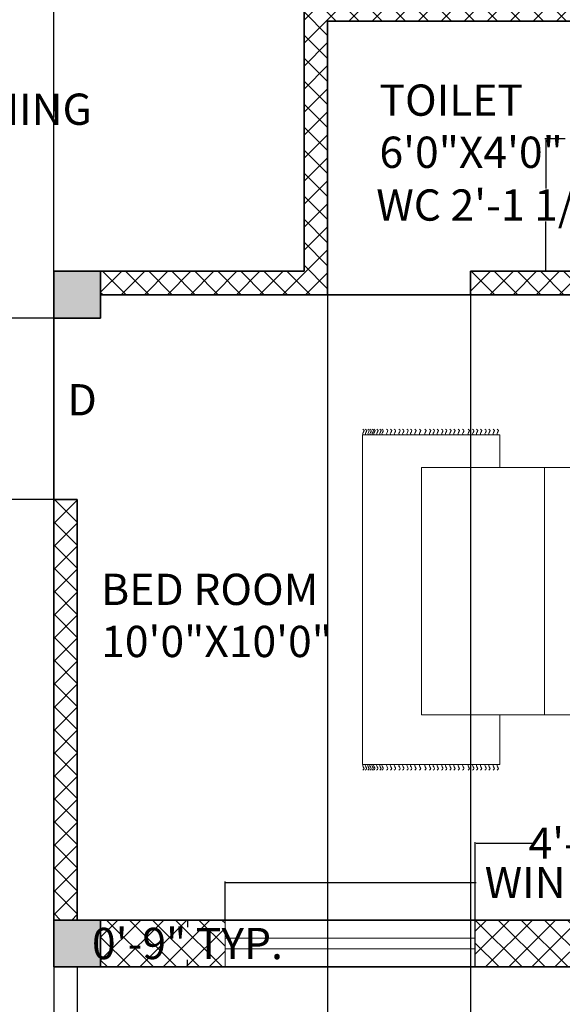
# Model space of a CAD drawing. Units: inches. Extents: x 958 to 1375, y 3152 to 3689.
# Tile 3 of 8: x 1167 to 1271, y 3251 to 3440. Entities that reach past the tile are written whole.
import ezdxf

# ---------------------------------------------------------------- set-up
doc = ezdxf.new("R2010")
doc.units = ezdxf.units.IN
doc.header["$MEASUREMENT"] = 0
for name, color, linetype, lineweight in [('A-ANNO-DIMS', 2, 'Continuous', 18), ('A-AREA-IDEN', 7, 'Continuous', 18), ('A-COLS', 7, 'Continuous', 35), ('A-DOOR-IDEN', 7, 'Continuous', 18), ('A-FURN', 8, 'Continuous', 18), ('A-WALL', 7, 'Continuous', 35), ('windows', 140, 'Continuous', 18)]:
    doc.layers.add(name, color=color, linetype=linetype, lineweight=lineweight)
doc.layers.add('A-COLS-PATT', color=18, linetype='Continuous', lineweight=13, true_color=0x000000)
doc.layers.add('A-WALL-PATT', color=240, linetype='Continuous', lineweight=13, true_color=0xed1f24)
doc.styles.get("Standard").update_dxf_attribs({"font": 'arial.ttf'})
doc.dimstyles.get("Standard").update_dxf_attribs({"dimtxt": 6, "dimasz": 0.18, "dimexe": 0.18, "dimexo": 0.0625, "dimgap": 0.09, "dimtad": 0, "dimtih": 1, "dimtoh": 1, "dimdec": 1, "dimzin": 0, "dimdsep": 46, "dimlunit": 3, "dimtxsty": 'Standard', "dimcen": 0.09, "dimadec": 0, "dimazin": 0, "dimtfac": 1, "dimtdec": 1, "dimtofl": 0, "dimtmove": 0, "dimatfit": 3, "dimfxl": 1, "dimtolj": 1, "dimtzin": 0, "dimarcsym": 0})

# ---------------------------------------------------------------- blocks, each defined once
blk = doc.blocks.new('*D9')
at = {"layer": 'A-ANNO-DIMS', "color": 0, "lineweight": -2, "transparency": 16777216}
for p, q in [((1177.7, 3257.97), (1177.7, 3236.74)), ((1297.7, 3257.97), (1297.7, 3236.74)), ((1177.88, 3236.92), (1232.8, 3236.92)), ((1297.52, 3236.92), (1242.6, 3236.92))]:
    blk.add_line(p, q, dxfattribs=at)
at = {"layer": 'A-ANNO-DIMS', "color": 0, "transparency": 16777216}
for points in [[(1177.88, 3236.95), (1177.88, 3236.89), (1177.7, 3236.92)], [(1297.52, 3236.95), (1297.52, 3236.89), (1297.7, 3236.92)]]:
    blk.add_solid(points, dxfattribs=at)
at = {"layer": 'Defpoints', "color": 0, "transparency": 16777216}
for p in [(1177.7, 3258.03), (1297.7, 3258.03), (1177.7, 3236.92)]:
    blk.add_point(p, dxfattribs=at)
at = {"layer": 'A-ANNO-DIMS', "color": 0, "transparency": 16777216, "insert": (1237.7, 3236.92), "char_height": 6, "attachment_point": 5}
blk.add_mtext("\\A1;10'", dxfattribs=at)
blk = doc.blocks.new('*D10')
at = {"layer": 'A-ANNO-DIMS', "color": 0, "lineweight": -2, "transparency": 16777216}
for p, q in [((1053.2, 3257.97), (1053.2, 3236.74)), ((1173.2, 3257.97), (1173.2, 3236.74)), ((1053.38, 3236.92), (1108.3, 3236.92)), ((1173.02, 3236.92), (1118.1, 3236.92))]:
    blk.add_line(p, q, dxfattribs=at)
at = {"layer": 'A-ANNO-DIMS', "color": 0, "transparency": 16777216}
for points in [[(1053.38, 3236.95), (1053.38, 3236.89), (1053.2, 3236.92)], [(1173.02, 3236.95), (1173.02, 3236.89), (1173.2, 3236.92)]]:
    blk.add_solid(points, dxfattribs=at)
at = {"layer": 'Defpoints', "color": 0, "transparency": 16777216}
for p in [(1053.2, 3258.03), (1173.2, 3258.03), (1173.2, 3236.92)]:
    blk.add_point(p, dxfattribs=at)
at = {"layer": 'A-ANNO-DIMS', "color": 0, "transparency": 16777216, "insert": (1113.2, 3236.92), "char_height": 6, "attachment_point": 5}
blk.add_mtext("\\A1;10'", dxfattribs=at)
blk = doc.blocks.new('BED-DOUBLE')
for p, q in [((5.6, 61.62), (5.6, 51.56)), ((63.65, 61.72), (63.65, 51.66)), ((68.68, 56.69), (58.62, 56.69)), ((10.63, 56.59), (0.57, 56.59)), ((49.39, 52.82), (10.63, 52.82)), ((49.44, 52), (10.63, 52)), ((49.39, 52.82), (58, 46.47)), ((49.44, 52.82), (49.44, 46.47)), ((49.44, 46.47), (58, 46.47)), ((58.05, 34.96), (10.63, 34.96)), ((4.36, 0), (4.36, 26.37)), ((4.36, 26.37), (10.65, 26.37)), ((58.05, 26.37), (67.59, 26.37)), ((67.59, 26.37), (67.59, 0)), ((67.59, 0), (4.36, 0))]:
    blk.add_line(p, q)
for points in [[(0, 50.39), (10.63, 50.5), (10.63, 62.68), (0, 62.58)], [(58.05, 62.68), (58.05, 11.37), (10.63, 11.37), (10.63, 62.68)], [(58.05, 50.5), (68.68, 50.6), (68.68, 62.78), (58.05, 62.68)], [(29.88, 59.98), (29.88, 52.82), (15.98, 52.82), (15.98, 59.98)], [(49.44, 59.98), (49.44, 52.82), (35.55, 52.82), (35.55, 59.98)]]:
    blk.add_lwpolyline(points, close=True)
for centre in [(5.6, 56.59), (63.65, 56.69)]:
    blk.add_circle(centre, 3.92)
for points, knots in [([(3.23, 25.84), (3.32, 25.96), (3.52, 26.2), (3.86, 25.96), (4.14, 25.78), (4.29, 25.89), (4.36, 25.94)], [0, 0, 0, 0, 0.400747, 0.791423, 1.067667, 1.29709, 1.29709, 1.29709, 1.29709]), ([(3.23, 25.06), (3.32, 25.18), (3.52, 25.42), (3.86, 25.18), (4.14, 25.01), (4.29, 25.11), (4.36, 25.16)], [0, 0, 0, 0, 0.400747, 0.791423, 1.067667, 1.29709, 1.29709, 1.29709, 1.29709]), ([(68.71, 25.84), (68.61, 25.96), (68.42, 26.2), (68.08, 25.96), (67.8, 25.78), (67.65, 25.89), (67.58, 25.94)], [0, 0, 0, 0, 0.400747, 0.791423, 1.067667, 1.29709, 1.29709, 1.29709, 1.29709]), ([(68.71, 25.06), (68.61, 25.18), (68.42, 25.42), (68.08, 25.18), (67.8, 25.01), (67.65, 25.11), (67.58, 25.16)], [0, 0, 0, 0, 0.400747, 0.791423, 1.067667, 1.29709, 1.29709, 1.29709, 1.29709]), ([(3.23, 24.24), (3.32, 24.36), (3.52, 24.6), (3.86, 24.36), (4.14, 24.19), (4.29, 24.3), (4.36, 24.34)], [0, 0, 0, 0, 0.400747, 0.791423, 1.067667, 1.29709, 1.29709, 1.29709, 1.29709]), ([(3.23, 23.51), (3.32, 23.63), (3.52, 23.87), (3.86, 23.63), (4.14, 23.46), (4.29, 23.57), (4.36, 23.62)], [0, 0, 0, 0, 0.400747, 0.791423, 1.067667, 1.29709, 1.29709, 1.29709, 1.29709]), ([(3.23, 22.63), (3.32, 22.75), (3.52, 22.99), (3.86, 22.75), (4.14, 22.58), (4.29, 22.69), (4.36, 22.73)], [0, 0, 0, 0, 0.400747, 0.791423, 1.067667, 1.29709, 1.29709, 1.29709, 1.29709]), ([(68.71, 24.24), (68.61, 24.36), (68.42, 24.6), (68.08, 24.36), (67.8, 24.19), (67.65, 24.3), (67.58, 24.34)], [0, 0, 0, 0, 0.400747, 0.791423, 1.067667, 1.29709, 1.29709, 1.29709, 1.29709]), ([(68.71, 23.51), (68.61, 23.63), (68.42, 23.87), (68.08, 23.63), (67.8, 23.46), (67.65, 23.57), (67.58, 23.62)], [0, 0, 0, 0, 0.400747, 0.791423, 1.067667, 1.29709, 1.29709, 1.29709, 1.29709]), ([(68.71, 22.63), (68.61, 22.75), (68.42, 22.99), (68.08, 22.75), (67.8, 22.58), (67.65, 22.69), (67.58, 22.73)], [0, 0, 0, 0, 0.400747, 0.791423, 1.067667, 1.29709, 1.29709, 1.29709, 1.29709]), ([(3.23, 21.88), (3.32, 22), (3.52, 22.24), (3.86, 22), (4.14, 21.83), (4.29, 21.93), (4.36, 21.98)], [0, 0, 0, 0, 0.400747, 0.791423, 1.067667, 1.29709, 1.29709, 1.29709, 1.29709]), ([(3.23, 21.15), (3.32, 21.27), (3.52, 21.51), (3.86, 21.27), (4.14, 21.1), (4.29, 21.21), (4.36, 21.25)], [0, 0, 0, 0, 0.400747, 0.791423, 1.067667, 1.29709, 1.29709, 1.29709, 1.29709]), ([(68.71, 21.88), (68.61, 22), (68.42, 22.24), (68.08, 22), (67.8, 21.83), (67.65, 21.93), (67.58, 21.98)], [0, 0, 0, 0, 0.400747, 0.791423, 1.067667, 1.29709, 1.29709, 1.29709, 1.29709]), ([(68.71, 21.15), (68.61, 21.27), (68.42, 21.51), (68.08, 21.27), (67.8, 21.1), (67.65, 21.21), (67.58, 21.25)], [0, 0, 0, 0, 0.400747, 0.791423, 1.067667, 1.29709, 1.29709, 1.29709, 1.29709]), ([(3.23, 20.27), (3.32, 20.39), (3.52, 20.63), (3.86, 20.39), (4.14, 20.22), (4.29, 20.32), (4.36, 20.37)], [0, 0, 0, 0, 0.400747, 0.791423, 1.067667, 1.29709, 1.29709, 1.29709, 1.29709]), ([(3.23, 19.23), (3.32, 19.35), (3.52, 19.59), (3.86, 19.35), (4.14, 19.18), (4.29, 19.29), (4.36, 19.33)], [0, 0, 0, 0, 0.400747, 0.791423, 1.067667, 1.29709, 1.29709, 1.29709, 1.29709]), ([(68.71, 20.27), (68.61, 20.39), (68.42, 20.63), (68.08, 20.39), (67.8, 20.22), (67.65, 20.32), (67.58, 20.37)], [0, 0, 0, 0, 0.400747, 0.791423, 1.067667, 1.29709, 1.29709, 1.29709, 1.29709]), ([(68.71, 19.23), (68.61, 19.35), (68.42, 19.59), (68.08, 19.35), (67.8, 19.18), (67.65, 19.29), (67.58, 19.33)], [0, 0, 0, 0, 0.400747, 0.791423, 1.067667, 1.29709, 1.29709, 1.29709, 1.29709]), ([(3.23, 18.35), (3.32, 18.47), (3.52, 18.71), (3.86, 18.47), (4.14, 18.3), (4.29, 18.4), (4.36, 18.45)], [0, 0, 0, 0, 0.400747, 0.791423, 1.067667, 1.29709, 1.29709, 1.29709, 1.29709]), ([(3.23, 17.53), (3.32, 17.65), (3.52, 17.89), (3.86, 17.65), (4.14, 17.48), (4.29, 17.59), (4.36, 17.64)], [0, 0, 0, 0, 0.400747, 0.791423, 1.067667, 1.29709, 1.29709, 1.29709, 1.29709]), ([(3.23, 16.76), (3.32, 16.88), (3.52, 17.12), (3.86, 16.88), (4.14, 16.71), (4.29, 16.81), (4.36, 16.86)], [0, 0, 0, 0, 0.400747, 0.791423, 1.067667, 1.29709, 1.29709, 1.29709, 1.29709]), ([(68.71, 18.35), (68.61, 18.47), (68.42, 18.71), (68.08, 18.47), (67.8, 18.3), (67.65, 18.4), (67.58, 18.45)], [0, 0, 0, 0, 0.400747, 0.791423, 1.067667, 1.29709, 1.29709, 1.29709, 1.29709]), ([(68.71, 17.53), (68.61, 17.65), (68.42, 17.89), (68.08, 17.65), (67.8, 17.48), (67.65, 17.59), (67.58, 17.64)], [0, 0, 0, 0, 0.400747, 0.791423, 1.067667, 1.29709, 1.29709, 1.29709, 1.29709]), ([(68.71, 16.76), (68.61, 16.88), (68.42, 17.12), (68.08, 16.88), (67.8, 16.71), (67.65, 16.81), (67.58, 16.86)], [0, 0, 0, 0, 0.400747, 0.791423, 1.067667, 1.29709, 1.29709, 1.29709, 1.29709]), ([(3.23, 15.94), (3.32, 16.06), (3.52, 16.3), (3.86, 16.06), (4.14, 15.89), (4.29, 16), (4.36, 16.04)], [0, 0, 0, 0, 0.400747, 0.791423, 1.067667, 1.29709, 1.29709, 1.29709, 1.29709]), ([(3.23, 15.21), (3.32, 15.33), (3.52, 15.57), (3.86, 15.33), (4.14, 15.16), (4.29, 15.27), (4.36, 15.32)], [0, 0, 0, 0, 0.400747, 0.791423, 1.067667, 1.29709, 1.29709, 1.29709, 1.29709]), ([(68.71, 15.94), (68.61, 16.06), (68.42, 16.3), (68.08, 16.06), (67.8, 15.89), (67.65, 16), (67.58, 16.04)], [0, 0, 0, 0, 0.400747, 0.791423, 1.067667, 1.29709, 1.29709, 1.29709, 1.29709]), ([(68.71, 15.21), (68.61, 15.33), (68.42, 15.57), (68.08, 15.33), (67.8, 15.16), (67.65, 15.27), (67.58, 15.32)], [0, 0, 0, 0, 0.400747, 0.791423, 1.067667, 1.29709, 1.29709, 1.29709, 1.29709]), ([(3.23, 14.33), (3.32, 14.45), (3.52, 14.69), (3.86, 14.45), (4.14, 14.28), (4.29, 14.39), (4.36, 14.43)], [0, 0, 0, 0, 0.400747, 0.791423, 1.067667, 1.29709, 1.29709, 1.29709, 1.29709]), ([(3.23, 13.58), (3.32, 13.7), (3.52, 13.94), (3.86, 13.7), (4.14, 13.53), (4.29, 13.63), (4.36, 13.68)], [0, 0, 0, 0, 0.400747, 0.791423, 1.067667, 1.29709, 1.29709, 1.29709, 1.29709]), ([(68.71, 14.33), (68.61, 14.45), (68.42, 14.69), (68.08, 14.45), (67.8, 14.28), (67.65, 14.39), (67.58, 14.43)], [0, 0, 0, 0, 0.400747, 0.791423, 1.067667, 1.29709, 1.29709, 1.29709, 1.29709]), ([(68.71, 13.58), (68.61, 13.7), (68.42, 13.94), (68.08, 13.7), (67.8, 13.53), (67.65, 13.63), (67.58, 13.68)], [0, 0, 0, 0, 0.400747, 0.791423, 1.067667, 1.29709, 1.29709, 1.29709, 1.29709]), ([(3.23, 12.85), (3.32, 12.97), (3.52, 13.21), (3.86, 12.97), (4.14, 12.8), (4.29, 12.9), (4.36, 12.95)], [0, 0, 0, 0, 0.400747, 0.791423, 1.067667, 1.29709, 1.29709, 1.29709, 1.29709]), ([(3.23, 11.97), (3.32, 12.09), (3.52, 12.33), (3.86, 12.09), (4.14, 11.92), (4.29, 12.02), (4.36, 12.07)], [0, 0, 0, 0, 0.400747, 0.791423, 1.067667, 1.29709, 1.29709, 1.29709, 1.29709]), ([(68.71, 12.85), (68.61, 12.97), (68.42, 13.21), (68.08, 12.97), (67.8, 12.8), (67.65, 12.9), (67.58, 12.95)], [0, 0, 0, 0, 0.400747, 0.791423, 1.067667, 1.29709, 1.29709, 1.29709, 1.29709]), ([(68.71, 11.97), (68.61, 12.09), (68.42, 12.33), (68.08, 12.09), (67.8, 11.92), (67.65, 12.02), (67.58, 12.07)], [0, 0, 0, 0, 0.400747, 0.791423, 1.067667, 1.29709, 1.29709, 1.29709, 1.29709]), ([(3.23, 10.93), (3.32, 11.05), (3.52, 11.29), (3.86, 11.05), (4.14, 10.88), (4.29, 10.99), (4.36, 11.03)], [0, 0, 0, 0, 0.400747, 0.791423, 1.067667, 1.29709, 1.29709, 1.29709, 1.29709]), ([(3.23, 10.05), (3.32, 10.17), (3.52, 10.41), (3.86, 10.17), (4.14, 10), (4.29, 10.1), (4.36, 10.15)], [0, 0, 0, 0, 0.400747, 0.791423, 1.067667, 1.29709, 1.29709, 1.29709, 1.29709]), ([(3.23, 9.23), (3.32, 9.35), (3.52, 9.59), (3.86, 9.35), (4.14, 9.18), (4.29, 9.29), (4.36, 9.34)], [0, 0, 0, 0, 0.400747, 0.791423, 1.067667, 1.29709, 1.29709, 1.29709, 1.29709]), ([(68.71, 10.93), (68.61, 11.05), (68.42, 11.29), (68.08, 11.05), (67.8, 10.88), (67.65, 10.99), (67.58, 11.03)], [0, 0, 0, 0, 0.400747, 0.791423, 1.067667, 1.29709, 1.29709, 1.29709, 1.29709]), ([(68.71, 10.05), (68.61, 10.17), (68.42, 10.41), (68.08, 10.17), (67.8, 10), (67.65, 10.1), (67.58, 10.15)], [0, 0, 0, 0, 0.400747, 0.791423, 1.067667, 1.29709, 1.29709, 1.29709, 1.29709]), ([(68.71, 9.23), (68.61, 9.35), (68.42, 9.59), (68.08, 9.35), (67.8, 9.18), (67.65, 9.29), (67.58, 9.34)], [0, 0, 0, 0, 0.400747, 0.791423, 1.067667, 1.29709, 1.29709, 1.29709, 1.29709]), ([(3.23, 8.54), (3.32, 8.66), (3.52, 8.9), (3.86, 8.66), (4.14, 8.49), (4.29, 8.6), (4.36, 8.65)], [0, 0, 0, 0, 0.400747, 0.791423, 1.067667, 1.29709, 1.29709, 1.29709, 1.29709]), ([(3.23, 7.73), (3.32, 7.85), (3.52, 8.09), (3.86, 7.85), (4.14, 7.68), (4.29, 7.78), (4.36, 7.83)], [0, 0, 0, 0, 0.400747, 0.791423, 1.067667, 1.29709, 1.29709, 1.29709, 1.29709]), ([(68.71, 8.54), (68.61, 8.66), (68.42, 8.9), (68.08, 8.66), (67.8, 8.49), (67.65, 8.6), (67.58, 8.65)], [0, 0, 0, 0, 0.400747, 0.791423, 1.067667, 1.29709, 1.29709, 1.29709, 1.29709]), ([(68.71, 7.73), (68.61, 7.85), (68.42, 8.09), (68.08, 7.85), (67.8, 7.68), (67.65, 7.78), (67.58, 7.83)], [0, 0, 0, 0, 0.400747, 0.791423, 1.067667, 1.29709, 1.29709, 1.29709, 1.29709]), ([(3.23, 7), (3.32, 7.12), (3.52, 7.36), (3.86, 7.12), (4.14, 6.95), (4.29, 7.05), (4.36, 7.1)], [0, 0, 0, 0, 0.400747, 0.791423, 1.067667, 1.29709, 1.29709, 1.29709, 1.29709]), ([(3.23, 6.12), (3.32, 6.24), (3.52, 6.48), (3.86, 6.24), (4.14, 6.07), (4.29, 6.17), (4.36, 6.22)], [0, 0, 0, 0, 0.400747, 0.791423, 1.067667, 1.29709, 1.29709, 1.29709, 1.29709]), ([(68.71, 7), (68.61, 7.12), (68.42, 7.36), (68.08, 7.12), (67.8, 6.95), (67.65, 7.05), (67.58, 7.1)], [0, 0, 0, 0, 0.400747, 0.791423, 1.067667, 1.29709, 1.29709, 1.29709, 1.29709]), ([(68.71, 6.12), (68.61, 6.24), (68.42, 6.48), (68.08, 6.24), (67.8, 6.07), (67.65, 6.17), (67.58, 6.22)], [0, 0, 0, 0, 0.400747, 0.791423, 1.067667, 1.29709, 1.29709, 1.29709, 1.29709]), ([(3.23, 5.37), (3.32, 5.49), (3.52, 5.73), (3.86, 5.49), (4.14, 5.31), (4.29, 5.42), (4.36, 5.47)], [0, 0, 0, 0, 0.400747, 0.791423, 1.067667, 1.29709, 1.29709, 1.29709, 1.29709]), ([(3.23, 4.64), (3.32, 4.76), (3.52, 5), (3.86, 4.76), (4.14, 4.59), (4.29, 4.69), (4.36, 4.74)], [0, 0, 0, 0, 0.400747, 0.791423, 1.067667, 1.29709, 1.29709, 1.29709, 1.29709]), ([(3.23, 3.75), (3.32, 3.88), (3.52, 4.12), (3.86, 3.88), (4.14, 3.7), (4.29, 3.81), (4.36, 3.86)], [0, 0, 0, 0, 0.400747, 0.791423, 1.067667, 1.29709, 1.29709, 1.29709, 1.29709]), ([(68.71, 5.37), (68.61, 5.49), (68.42, 5.73), (68.08, 5.49), (67.8, 5.31), (67.65, 5.42), (67.58, 5.47)], [0, 0, 0, 0, 0.400747, 0.791423, 1.067667, 1.29709, 1.29709, 1.29709, 1.29709]), ([(68.71, 4.64), (68.61, 4.76), (68.42, 5), (68.08, 4.76), (67.8, 4.59), (67.66, 4.69), (67.59, 4.73)], [0, 0, 0, 0, 0.400747, 0.791423, 1.067667, 1.283686, 1.283686, 1.283686, 1.283686]), ([(68.71, 3.75), (68.61, 3.88), (68.42, 4.12), (68.08, 3.88), (67.8, 3.7), (67.66, 3.81), (67.59, 3.85)], [0, 0, 0, 0, 0.400747, 0.791423, 1.067667, 1.283686, 1.283686, 1.283686, 1.283686]), ([(3.23, 3.33), (3.32, 3.45), (3.52, 3.7), (3.86, 3.45), (4.14, 3.27), (4.29, 3.38), (4.36, 3.43)], [0, 0, 0, 0, 0.407265, 0.802015, 1.07826, 1.307683, 1.307683, 1.307683, 1.307683]), ([(3.23, 2.76), (3.32, 2.88), (3.52, 3.12), (3.86, 2.88), (4.14, 2.71), (4.29, 2.81), (4.36, 2.86)], [0, 0, 0, 0, 0.400747, 0.791423, 1.067667, 1.29709, 1.29709, 1.29709, 1.29709]), ([(3.23, 2.19), (3.32, 2.31), (3.52, 2.55), (3.86, 2.31), (4.14, 2.13), (4.29, 2.24), (4.36, 2.29)], [0, 0, 0, 0, 0.400747, 0.791423, 1.067667, 1.29709, 1.29709, 1.29709, 1.29709]), ([(3.23, 1.88), (3.32, 2), (3.52, 2.24), (3.86, 2), (4.14, 1.82), (4.29, 1.93), (4.36, 1.98)], [0, 0, 0, 0, 0.400747, 0.791423, 1.067667, 1.29709, 1.29709, 1.29709, 1.29709]), ([(68.71, 3.33), (68.61, 3.45), (68.42, 3.69), (68.08, 3.45), (67.8, 3.28), (67.66, 3.38), (67.59, 3.42)], [0, 0, 0, 0, 0.402903, 0.794912, 1.071156, 1.287177, 1.287177, 1.287177, 1.287177]), ([(68.71, 2.73), (68.61, 2.85), (68.42, 3.09), (68.08, 2.85), (67.8, 2.68), (67.66, 2.78), (67.59, 2.83)], [0, 0, 0, 0, 0.400747, 0.791423, 1.067667, 1.283686, 1.283686, 1.283686, 1.283686]), ([(68.71, 2.16), (68.61, 2.28), (68.42, 2.52), (68.08, 2.28), (67.8, 2.11), (67.66, 2.21), (67.59, 2.25)], [0, 0, 0, 0, 0.400747, 0.791423, 1.067667, 1.283686, 1.283686, 1.283686, 1.283686]), ([(68.71, 1.85), (68.61, 1.97), (68.42, 2.21), (68.08, 1.97), (67.8, 1.8), (67.66, 1.9), (67.59, 1.94)], [0, 0, 0, 0, 0.400747, 0.791423, 1.067667, 1.283686, 1.283686, 1.283686, 1.283686]), ([(3.23, 1.46), (3.32, 1.58), (3.52, 1.82), (3.86, 1.58), (4.14, 1.41), (4.29, 1.51), (4.36, 1.56)], [0, 0, 0, 0, 0.400747, 0.791423, 1.067667, 1.29709, 1.29709, 1.29709, 1.29709]), ([(3.23, 1.06), (3.32, 1.18), (3.52, 1.42), (3.86, 1.18), (4.14, 1.01), (4.29, 1.11), (4.36, 1.16)], [0, 0, 0, 0, 0.400747, 0.791423, 1.067667, 1.29709, 1.29709, 1.29709, 1.29709]), ([(3.23, 0.57), (3.32, 0.7), (3.52, 0.94), (3.86, 0.7), (4.14, 0.52), (4.29, 0.63), (4.36, 0.68)], [0, 0, 0, 0, 0.400747, 0.791423, 1.067667, 1.29709, 1.29709, 1.29709, 1.29709]), ([(3.23, 0.07), (3.32, 0.19), (3.52, 0.43), (3.86, 0.19), (4.14, 0.02), (4.29, 0.13), (4.36, 0.18)], [0, 0, 0, 0, 0.400747, 0.791423, 1.067667, 1.29709, 1.29709, 1.29709, 1.29709]), ([(68.71, 1.43), (68.61, 1.55), (68.42, 1.79), (68.08, 1.55), (67.8, 1.38), (67.65, 1.48), (67.58, 1.53)], [0, 0, 0, 0, 0.400747, 0.791423, 1.067667, 1.29709, 1.29709, 1.29709, 1.29709]), ([(68.71, 1.03), (68.61, 1.15), (68.42, 1.39), (68.08, 1.15), (67.8, 0.98), (67.65, 1.09), (67.58, 1.13)], [0, 0, 0, 0, 0.400747, 0.791423, 1.067667, 1.29709, 1.29709, 1.29709, 1.29709]), ([(68.71, 0.55), (68.61, 0.67), (68.42, 0.91), (68.08, 0.67), (67.8, 0.5), (67.65, 0.6), (67.58, 0.65)], [0, 0, 0, 0, 0.400747, 0.791423, 1.067667, 1.29709, 1.29709, 1.29709, 1.29709]), ([(68.71, 0.07), (68.61, 0.19), (68.42, 0.43), (68.08, 0.19), (67.8, 0.02), (67.65, 0.13), (67.58, 0.18)], [0, 0, 0, 0, 0.400747, 0.791423, 1.067667, 1.29709, 1.29709, 1.29709, 1.29709])]:
    blk.add_open_spline(points, degree=3, knots=knots)
blk = doc.blocks.new('WIN-48')
for p, q in [((48, 9), (0, 9)), ((48, 5.5), (0, 5.5)), ((0, 3.5), (48, 3.5)), ((0, 0), (48, 0))]:
    blk.add_line(p, q)
blk = doc.blocks.new('*D22')
at = {"layer": 'A-ANNO-DIMS', "color": 0, "lineweight": -2, "transparency": 16777216}
for p, q in [((1206.05, 3267.1), (1206.05, 3274.41)), ((1206.23, 3274.23), (1253.87, 3274.23)), ((1254.05, 3267.1), (1254.05, 3274.41)), ((1254.05, 3274.23), (1254.23, 3274.23))]:
    blk.add_line(p, q, dxfattribs=at)
at = {"layer": 'A-ANNO-DIMS', "color": 0, "transparency": 16777216}
for points in [[(1206.23, 3274.26), (1206.23, 3274.2), (1206.05, 3274.23)], [(1253.87, 3274.26), (1253.87, 3274.2), (1254.05, 3274.23)]]:
    blk.add_solid(points, dxfattribs=at)
at = {"layer": 'Defpoints', "color": 0, "transparency": 16777216}
for p in [(1254.05, 3274.23), (1206.05, 3267.03), (1254.05, 3267.03)]:
    blk.add_point(p, dxfattribs=at)
at = {"layer": 'A-ANNO-DIMS', "color": 0, "transparency": 16777216, "insert": (1292.28, 3274.23), "char_height": 6, "attachment_point": 5}
blk.add_mtext('\\A1;WINDOW 4\'-0" TYP.', dxfattribs=at)
blk = doc.blocks.new('*D23')
at = {"layer": 'A-ANNO-DIMS', "color": 0, "lineweight": -2, "transparency": 16777216}
for p, q in [((1205.99, 3267.03), (1198.67, 3267.03)), ((1198.85, 3266.85), (1198.85, 3265.69)), ((1205.99, 3258.03), (1198.67, 3258.03)), ((1198.85, 3258.21), (1198.85, 3259.38))]:
    blk.add_line(p, q, dxfattribs=at)
at = {"layer": 'A-ANNO-DIMS', "color": 0, "transparency": 16777216}
for points in [[(1198.82, 3266.85), (1198.88, 3266.85), (1198.85, 3267.03)], [(1198.82, 3258.21), (1198.88, 3258.21), (1198.85, 3258.03)]]:
    blk.add_solid(points, dxfattribs=at)
at = {"layer": 'Defpoints', "color": 0, "transparency": 16777216}
for p in [(1198.85, 3267.03), (1206.05, 3267.03), (1206.05, 3258.03)]:
    blk.add_point(p, dxfattribs=at)
at = {"layer": 'A-ANNO-DIMS', "color": 0, "transparency": 16777216, "insert": (1198.85, 3262.53), "char_height": 6, "attachment_point": 5}
blk.add_mtext('\\A1;0\'-9" TYP.', dxfattribs=at)
blk = doc.blocks.new('*D28')
at = {"layer": 'A-ANNO-DIMS', "color": 0, "lineweight": -2, "transparency": 16777216}
for p, q in [((1271.31, 3416.95), (1267.38, 3416.95)), ((1267.56, 3416.77), (1267.56, 3407.43)), ((1267.56, 3391.72), (1267.56, 3401.05)), ((1271.31, 3391.54), (1267.38, 3391.54))]:
    blk.add_line(p, q, dxfattribs=at)
at = {"layer": 'A-ANNO-DIMS', "color": 0, "transparency": 16777216}
for points in [[(1267.53, 3416.77), (1267.59, 3416.77), (1267.56, 3416.95)], [(1267.53, 3391.72), (1267.59, 3391.72), (1267.56, 3391.54)]]:
    blk.add_solid(points, dxfattribs=at)
at = {"layer": 'Defpoints', "color": 0, "transparency": 16777216}
for p in [(1267.56, 3416.95), (1271.38, 3416.95), (1271.38, 3391.54)]:
    blk.add_point(p, dxfattribs=at)
at = {"layer": 'A-ANNO-DIMS', "color": 0, "transparency": 16777216, "insert": (1267.56, 3404.24), "char_height": 6, "attachment_point": 5}
blk.add_mtext('\\A1;WC 2\'-1 1/2" TYP.', dxfattribs=at)
blk = doc.blocks.new('*D32')
at = {"layer": 'A-ANNO-DIMS', "color": 0, "lineweight": -2, "transparency": 16777216}
for p, q in [((1115.92, 3446.28), (1115.92, 3448.44)), ((1129.61, 3446.28), (1129.61, 3448.44)), ((1116.1, 3448.26), (1129.43, 3448.26)), ((1129.61, 3448.26), (1129.79, 3448.26))]:
    blk.add_line(p, q, dxfattribs=at)
at = {"layer": 'A-ANNO-DIMS', "color": 0, "transparency": 16777216}
for points in [[(1116.1, 3448.29), (1116.1, 3448.23), (1115.92, 3448.26)], [(1129.43, 3448.29), (1129.43, 3448.23), (1129.61, 3448.26)]]:
    blk.add_solid(points, dxfattribs=at)
at = {"layer": 'Defpoints', "color": 0, "transparency": 16777216}
for p in [(1129.61, 3448.26), (1115.92, 3446.21), (1129.61, 3446.21)]:
    blk.add_point(p, dxfattribs=at)
at = {"layer": 'A-ANNO-DIMS', "color": 0, "transparency": 16777216, "insert": (1188.42, 3448.26), "char_height": 6, "attachment_point": 5}
blk.add_mtext('\\A1;CHAIR PROFILE 1\'-1 1/2" TYP.', dxfattribs=at)
blk = doc.blocks.new('*D44')
at = {"layer": 'A-ANNO-DIMS', "color": 0, "lineweight": -2, "transparency": 16777216}
for p, q in [((1132.32, 3267.1), (1132.32, 3649.46)), ((1132.5, 3649.28), (1144.69, 3649.28)), ((1173.02, 3649.28), (1160.82, 3649.28)), ((1173.2, 3267.1), (1173.2, 3649.46))]:
    blk.add_line(p, q, dxfattribs=at)
at = {"layer": 'A-ANNO-DIMS', "color": 0, "transparency": 16777216}
for points in [[(1132.5, 3649.31), (1132.5, 3649.25), (1132.32, 3649.28)], [(1173.02, 3649.31), (1173.02, 3649.25), (1173.2, 3649.28)]]:
    blk.add_solid(points, dxfattribs=at)
at = {"layer": 'Defpoints', "color": 0, "transparency": 16777216}
for p in [(1173.2, 3649.28), (1132.32, 3267.03), (1173.2, 3267.03)]:
    blk.add_point(p, dxfattribs=at)
at = {"layer": 'A-ANNO-DIMS', "color": 0, "transparency": 16777216, "insert": (1152.76, 3649.28), "char_height": 6, "attachment_point": 5}
blk.add_mtext('\\A1;3\'-5"', dxfattribs=at)
blk = doc.blocks.new('*D45')
at = {"layer": 'A-ANNO-DIMS', "color": 0, "lineweight": -2, "transparency": 16777216}
for p, q in [((1173.13, 3382.53), (1149.27, 3382.53)), ((1149.45, 3382.35), (1149.45, 3368.24)), ((1149.45, 3347.92), (1149.45, 3362.04)), ((1173.13, 3347.74), (1149.27, 3347.74))]:
    blk.add_line(p, q, dxfattribs=at)
at = {"layer": 'A-ANNO-DIMS', "color": 0, "transparency": 16777216}
for points in [[(1149.42, 3382.35), (1149.48, 3382.35), (1149.45, 3382.53)], [(1149.42, 3347.92), (1149.48, 3347.92), (1149.45, 3347.74)]]:
    blk.add_solid(points, dxfattribs=at)
at = {"layer": 'Defpoints', "color": 0, "transparency": 16777216}
for p in [(1149.45, 3382.53), (1173.2, 3382.53), (1173.2, 3347.74)]:
    blk.add_point(p, dxfattribs=at)
at = {"layer": 'A-ANNO-DIMS', "color": 0, "transparency": 16777216, "insert": (1149.45, 3365.14), "char_height": 6, "attachment_point": 5}
blk.add_mtext('\\A1;2\'-11"', dxfattribs=at)
blk = doc.blocks.new('*D49')
at = {"layer": 'A-ANNO-DIMS', "color": 0, "lineweight": -2, "transparency": 16777216}
for p, q in [((1225.7, 3386.97), (1225.7, 3234.1)), ((1253.12, 3386.97), (1253.12, 3234.1)), ((1225.88, 3234.28), (1252.94, 3234.28)), ((1253.12, 3234.28), (1253.3, 3234.28))]:
    blk.add_line(p, q, dxfattribs=at)
at = {"layer": 'A-ANNO-DIMS', "color": 0, "transparency": 16777216}
for points in [[(1225.88, 3234.31), (1225.88, 3234.25), (1225.7, 3234.28)], [(1252.94, 3234.31), (1252.94, 3234.25), (1253.12, 3234.28)]]:
    blk.add_solid(points, dxfattribs=at)
at = {"layer": 'Defpoints', "color": 0, "transparency": 16777216}
for p in [(1225.7, 3387.03), (1253.12, 3387.03), (1253.12, 3234.28)]:
    blk.add_point(p, dxfattribs=at)
at = {"layer": 'A-ANNO-DIMS', "color": 0, "transparency": 16777216, "insert": (1268.4, 3234.28), "char_height": 6, "attachment_point": 5}
blk.add_mtext('\\A1;2\'-3 1/2"', dxfattribs=at)
blk = doc.blocks.new('*D54')
at = {"layer": 'A-ANNO-DIMS', "color": 0, "lineweight": -2, "transparency": 16777216}
for p, q in [((1254.05, 3258.1), (1254.05, 3281.96)), ((1254.23, 3281.78), (1265.2, 3281.78)), ((1306.52, 3281.78), (1295.55, 3281.78)), ((1306.7, 3258.1), (1306.7, 3281.96))]:
    blk.add_line(p, q, dxfattribs=at)
at = {"layer": 'A-ANNO-DIMS', "color": 0, "transparency": 16777216}
for points in [[(1254.23, 3281.81), (1254.23, 3281.75), (1254.05, 3281.78)], [(1306.52, 3281.81), (1306.52, 3281.75), (1306.7, 3281.78)]]:
    blk.add_solid(points, dxfattribs=at)
at = {"layer": 'Defpoints', "color": 0, "transparency": 16777216}
for p in [(1306.7, 3281.78), (1254.05, 3258.03), (1306.7, 3258.03)]:
    blk.add_point(p, dxfattribs=at)
at = {"layer": 'A-ANNO-DIMS', "color": 0, "transparency": 16777216, "insert": (1280.37, 3281.78), "char_height": 6, "attachment_point": 5}
blk.add_mtext('\\A1;4\'-4 1/2"', dxfattribs=at)
blk = doc.blocks.new('*D60')
at = {"layer": 'A-ANNO-DIMS', "color": 0, "lineweight": -2, "transparency": 16777216}
for p, q in [((1135.31, 3386.97), (1135.31, 3234.1)), ((1173.2, 3386.97), (1173.2, 3234.1)), ((1135.49, 3234.28), (1146.19, 3234.28)), ((1173.02, 3234.28), (1162.32, 3234.28))]:
    blk.add_line(p, q, dxfattribs=at)
at = {"layer": 'A-ANNO-DIMS', "color": 0, "transparency": 16777216}
for points in [[(1135.49, 3234.31), (1135.49, 3234.25), (1135.31, 3234.28)], [(1173.02, 3234.31), (1173.02, 3234.25), (1173.2, 3234.28)]]:
    blk.add_solid(points, dxfattribs=at)
at = {"layer": 'Defpoints', "color": 0, "transparency": 16777216}
for p in [(1135.31, 3387.03), (1173.2, 3387.03), (1173.2, 3234.28)]:
    blk.add_point(p, dxfattribs=at)
at = {"layer": 'A-ANNO-DIMS', "color": 0, "transparency": 16777216, "insert": (1154.25, 3234.28), "char_height": 6, "attachment_point": 5}
blk.add_mtext('\\A1;3\'-2"', dxfattribs=at)

msp = doc.modelspace()

# ---------------------------------------------------------------- hatches: boundary and pattern name
at = {"layer": 'A-COLS-PATT'}
h = msp.add_hatch(color=256, dxfattribs=at)
h.dxf.hatch_style = 1
h.paths.add_polyline_path([(1053.2, 3625.53), (1044.2, 3625.53), (1044.2, 3616.53), (1053.2, 3616.53)])
h.paths.add_polyline_path([(1182.2, 3625.53), (1173.2, 3625.53), (1173.2, 3616.53), (1182.2, 3616.53)])
h.paths.add_polyline_path([(1306.7, 3625.53), (1297.7, 3625.53), (1297.7, 3616.53), (1306.7, 3616.53)])
h.paths.add_polyline_path([(1306.7, 3501.03), (1297.7, 3501.03), (1297.7, 3492.03), (1306.7, 3492.03)])
h.paths.add_polyline_path([(1306.7, 3391.53), (1297.7, 3391.53), (1297.7, 3382.53), (1306.7, 3382.53)])
h.paths.add_polyline_path([(1306.7, 3267.03), (1297.7, 3267.03), (1297.7, 3258.03), (1306.7, 3258.03)])
h.paths.add_polyline_path([(1182.2, 3267.03), (1173.2, 3267.03), (1173.2, 3258.03), (1182.2, 3258.03)])
h.paths.add_polyline_path([(1053.2, 3267.03), (1044.2, 3267.03), (1044.2, 3258.03), (1053.2, 3258.03)])
h.paths.add_polyline_path([(1053.2, 3391.53), (1044.2, 3391.53), (1044.2, 3382.53), (1053.2, 3382.53)])
h.paths.add_polyline_path([(1053.2, 3501.03), (1044.2, 3501.03), (1044.2, 3492.03), (1053.2, 3492.03)])
h.paths.add_polyline_path([(1182.2, 3501.03), (1173.2, 3501.03), (1173.2, 3492.03), (1182.2, 3492.03)])
h.paths.add_polyline_path([(1182.2, 3391.53), (1173.2, 3391.53), (1173.2, 3382.53), (1182.2, 3382.53)])
at = {"layer": 'A-WALL-PATT'}
h = msp.add_hatch(dxfattribs=at)
h.set_pattern_fill('ANSI37', color=256, scale=25)
h.paths.add_polyline_path([(1080.68, 3625.53), (1053.2, 3625.53), (1053.2, 3616.53), (1080.68, 3616.53)])
h.paths.add_polyline_path([(1053.2, 3616.53), (1044.2, 3616.53), (1044.2, 3587.05), (1053.2, 3587.05)])
h.paths.add_polyline_path([(1173.2, 3625.53), (1128.68, 3625.53), (1128.68, 3616.53), (1173.2, 3616.53)])
h.paths.add_polyline_path([(1215.78, 3625.53), (1182.2, 3625.53), (1182.2, 3616.53), (1215.78, 3616.53)])
h.paths.add_polyline_path([(1297.7, 3625.53), (1263.78, 3625.53), (1263.78, 3616.53), (1297.7, 3616.53)])
h.paths.add_polyline_path([(1177.7, 3616.53), (1173.2, 3616.53), (1173.2, 3501.03), (1177.7, 3501.03)])
h.paths.add_polyline_path([(1053.2, 3539.05), (1044.2, 3539.05), (1044.2, 3501.03), (1053.2, 3501.03)])
h.paths.add_polyline_path([(1135.44, 3496.53), (1053.2, 3496.53), (1053.2, 3492.03), (1135.44, 3492.03)])
h.paths.add_polyline_path([(1306.7, 3616.53), (1297.7, 3616.53), (1297.7, 3586.38), (1306.7, 3586.38)])
h.paths.add_polyline_path([(1306.7, 3538.38), (1297.7, 3538.38), (1297.7, 3501.03), (1306.7, 3501.03)])
h.paths.add_polyline_path([(1297.7, 3496.53), (1216.84, 3496.53), (1216.84, 3492.03), (1297.7, 3492.03)])
h.paths.add_polyline_path([(1306.7, 3492.03), (1297.7, 3492.03), (1297.7, 3481.63), (1306.7, 3481.63)])
h.paths.add_polyline_path([(1306.7, 3457.63), (1297.7, 3457.63), (1297.7, 3444.03), (1225.7, 3444.03), (1225.7, 3462.51), (1221.2, 3462.51), (1221.2, 3391.53), (1182.2, 3391.53), (1182.2, 3387.03), (1225.7, 3387.03), (1225.7, 3439.53), (1297.7, 3439.53), (1297.7, 3428.57), (1306.7, 3428.57)])
h.paths.add_polyline_path([(1306.7, 3404.57), (1297.7, 3404.57), (1297.7, 3391.53), (1306.7, 3391.53)], flags=17)
h.paths.add_polyline_path([(1297.7, 3391.53), (1253.12, 3391.53), (1253.12, 3387.03), (1297.7, 3387.03)], flags=17)
h.paths.add_polyline_path([(1306.7, 3382.53), (1297.7, 3382.53), (1297.7, 3354.01), (1306.7, 3354.01)])
h.paths.add_polyline_path([(1306.7, 3306.01), (1297.7, 3306.01), (1297.7, 3267.03), (1306.7, 3267.03)])
h.paths.add_polyline_path([(1297.7, 3267.03), (1254.05, 3267.03), (1254.05, 3258.03), (1297.7, 3258.03)])
h.paths.add_polyline_path([(1177.7, 3347.74), (1173.2, 3347.74), (1173.2, 3267.03), (1177.7, 3267.03)])
h.paths.add_polyline_path([(1206.05, 3267.03), (1182.2, 3267.03), (1182.2, 3258.03), (1206.05, 3258.03)])
h.paths.add_polyline_path([(1053.2, 3308.96), (1044.2, 3308.96), (1044.2, 3267.03), (1053.2, 3267.03)])
h.paths.add_polyline_path([(1053.2, 3382.53), (1044.2, 3382.53), (1044.2, 3356.96), (1053.2, 3356.96)])
h.paths.add_polyline_path([(1053.2, 3420.58), (1044.2, 3420.58), (1044.2, 3391.53), (1053.2, 3391.53)])
h.paths.add_polyline_path([(1053.2, 3492.03), (1044.2, 3492.03), (1044.2, 3468.58), (1053.2, 3468.58)])

# ---------------------------------------------------------------- linework, layer by layer
at = {"layer": 'A-COLS'}
for p, q in [((1173.2, 3391.53), (1182.2, 3391.53)), ((1173.2, 3382.53), (1173.2, 3391.53)), ((1182.2, 3391.53), (1182.2, 3382.53)), ((1182.2, 3382.53), (1173.2, 3382.53)), ((1173.2, 3267.03), (1182.2, 3267.03)), ((1182.2, 3267.03), (1182.2, 3258.03)), ((1182.2, 3258.03), (1173.2, 3258.03))]:
    msp.add_line(p, q, dxfattribs=at)
at = {"layer": 'A-WALL'}
for p, q in [((1221.2, 3492.03), (1221.2, 3391.53)), ((1225.7, 3439.53), (1297.7, 3439.53)), ((1225.7, 3439.53), (1225.7, 3387.03)), ((1173.2, 3391.53), (1173.2, 3387.03)), ((1173.2, 3391.53), (1221.2, 3391.53)), ((1253.12, 3391.53), (1253.12, 3387.03)), ((1253.12, 3391.53), (1306.7, 3391.53)), ((1182.2, 3387.03), (1297.7, 3387.03)), ((1173.2, 3347.74), (1177.7, 3347.74)), ((1173.2, 3347.74), (1173.2, 3258.03)), ((1177.7, 3347.74), (1177.7, 3267.03)), ((1173.2, 3267.03), (1306.7, 3267.03)), ((1173.2, 3258.03), (1306.7, 3258.03))]:
    msp.add_line(p, q, dxfattribs=at)
at = {"layer": 'windows'}
for p, q in [((1206.05, 3267.03), (1206.05, 3258.03)), ((1254.05, 3258.03), (1254.05, 3267.03))]:
    msp.add_line(p, q, dxfattribs=at)

# ---------------------------------------------------------------- block references
at = {"layer": 'A-FURN', "rotation": 269.9999999999769}
msp.add_blockref('BED-DOUBLE', (1232.39, 3364.48), dxfattribs=at)
at = {"layer": 'windows'}
msp.add_blockref('WIN-48', (1206.05, 3258.03), dxfattribs=at)

# ---------------------------------------------------------------- texts
at = {"layer": 'A-AREA-IDEN', "char_height": 6, "attachment_point": 1}
for s, width, insert in [('KITCHEN / DINING\\P      14\'0"X8\'4"', 114.4555, (1111.24, 3425.63)), ('TOILET\\P6\'0"X4\'0"', 36.6599, (1235.67, 3427.37)), ('BED ROOM\\P10\'0"X10\'0"', 45.0029, (1182.3, 3333.49))]:
    msp.add_mtext_dynamic_manual_height_columns(s, width=width, gutter_width=1, heights=[0], dxfattribs=dict(at, insert=insert))
at = {"layer": 'A-DOOR-IDEN', "insert": (1175.84, 3369.87), "char_height": 6, "attachment_point": 1}
msp.add_mtext_dynamic_manual_height_columns('D ', width=17.9455, gutter_width=1, heights=[0], dxfattribs=at)

# ---------------------------------------------------------------- dimensions: what is measured, and where the dimension line sits
at = {"layer": 'A-ANNO-DIMS'}
for base, p1, p2, override, picture, middle in [((1173.2, 3649.28), (1132.32, 3267.03), (1173.2, 3267.03), {"dimdec": 1, "dimlfac": 1, "dimrnd": 0, "dimzin": 1, "dimdsep": 46, "dimlunit": 4, "dimfrac": 2}, '*D44', (1152.76, 3649.28)), ((1173.2, 3234.28), (1135.31, 3387.03), (1173.2, 3387.03), {"dimdec": 1, "dimlfac": 1, "dimrnd": 0, "dimzin": 1, "dimdsep": 46, "dimlunit": 4, "dimfrac": 2}, '*D60', (1154.25, 3234.28)), ((1253.12, 3234.28), (1225.7, 3387.03), (1253.12, 3387.03), {"dimdec": 1, "dimlfac": 1, "dimrnd": 0, "dimzin": 1, "dimdsep": 46, "dimlunit": 4, "dimfrac": 2}, '*D49', (1268.4, 3234.28)), ((1173.2, 3236.92), (1053.2, 3258.03), (1173.2, 3258.03), {"dimclrd": 0, "dimclre": 0, "dimclrt": 0}, '*D10', (1113.2, 3236.92)), ((1177.7, 3236.92), (1297.7, 3258.03), (1177.7, 3258.03), {"dimclrd": 0, "dimclre": 0, "dimclrt": 0}, '*D9', (1237.7, 3236.92))]:
    dim = msp.add_linear_dim(base=base, p1=p1, p2=p2, dimstyle='Standard', override=override, dxfattribs=at)
    dim.commit()
    dim.dimension.update_dxf_attribs({"geometry": picture, "text_midpoint": middle})
for base, p1, p2, text, picture, middle in [((1129.61, 3448.26), (1115.92, 3446.21), (1129.61, 3446.21), 'CHAIR PROFILE <> TYP.', '*D32', (1188.42, 3448.26)), ((1254.05, 3274.23), (1206.05, 3267.03), (1254.05, 3267.03), 'WINDOW <> TYP.', '*D22', (1292.28, 3274.23))]:
    dim = msp.add_linear_dim(base=base, p1=p1, p2=p2, text=text, dimstyle='Standard', override={"dimdec": 1, "dimlfac": 1, "dimrnd": 0, "dimzin": 1, "dimdsep": 46, "dimlunit": 4, "dimfrac": 2}, dxfattribs=at)
    dim.commit()
    dim.dimension.update_dxf_attribs({"geometry": picture, "text_midpoint": middle})
for base, p1, p2, text, picture, middle in [((1267.56, 3416.95), (1271.38, 3391.54), (1271.38, 3416.95), 'WC <> TYP.', '*D28', (1267.56, 3404.24)), ((1198.85, 3267.03), (1206.05, 3258.03), (1206.05, 3267.03), '<> TYP.', '*D23', (1198.85, 3262.53))]:
    dim = msp.add_linear_dim(base=base, p1=p1, p2=p2, angle=90, text=text, dimstyle='Standard', override={"dimdec": 1, "dimlfac": 1, "dimrnd": 0, "dimzin": 1, "dimdsep": 46, "dimlunit": 4, "dimfrac": 2}, dxfattribs=at)
    dim.commit()
    dim.dimension.update_dxf_attribs({"geometry": picture, "text_midpoint": middle})
for base, p1, p2, angle, picture, middle in [((1149.45, 3382.53), (1173.2, 3347.74), (1173.2, 3382.53), 90, '*D45', (1149.45, 3365.14)), ((1306.6972, 3281.7849), (1254.0507, 3258.0349), (1306.6972, 3258.0349), 0, '*D54', (1280.3739, 3281.7849))]:
    dim = msp.add_linear_dim(base=base, p1=p1, p2=p2, angle=angle, dimstyle='Standard', override={"dimdec": 1, "dimlfac": 1, "dimrnd": 0, "dimzin": 1, "dimdsep": 46, "dimlunit": 4, "dimfrac": 2}, dxfattribs=at)
    dim.commit()
    dim.dimension.update_dxf_attribs({"geometry": picture, "text_midpoint": middle})

doc.saveas('drawing.dxf')
